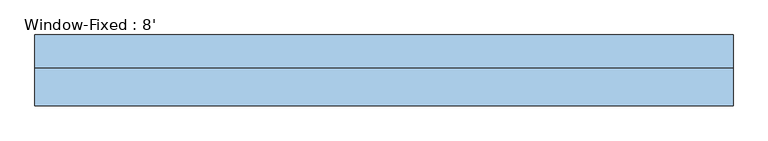
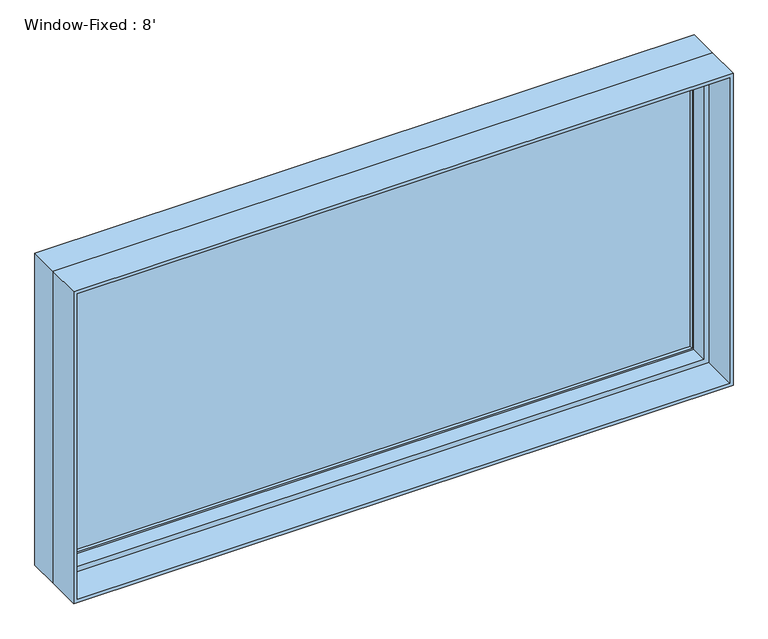
"""IFC4 building model written with IfcOpenShell, lengths in millimetres: window geometry, Window-Fixed : 8'."""

from ifc_helpers import new_model, si_unit, frame, origin, place, context, project, spatial, polyline, outline, extrude, faceted_brep, source, transform, mapped, element, save


def window_fixed_8_9704bb16(model_context):
    return source(origin(), model_context, "Body", "SolidModel", [
        faceted_brep([(1219.2, 19.05, 2133.6), (1219.2, 133.35, 2133.6), (-1219.2, 133.35, 2133.6), (-1219.2, 19.05, 2133.6), (-1219.2, 133.35, 914.4), (-1219.2, 19.05, 914.4), (1219.2, 133.35, 914.4), (1219.2, 19.05, 914.4), (1187.45, 19.05, 2101.85), (1187.45, 19.05, 946.15), (-1187.45, 19.05, 946.15), (-1187.45, 19.05, 2101.85), (-1206.5, 133.35, 2120.9), (-1206.5, 133.35, 927.1), (1206.5, 133.35, 927.1), (1206.5, 133.35, 2120.9), (1187.45, 82.55, 2101.85), (-1187.45, 82.55, 2101.85), (1206.5, 82.55, 2120.9), (-1206.5, 82.55, 2120.9), (-1187.45, 82.55, 946.15), (-1206.5, 82.55, 927.1), (1187.45, 82.55, 946.15), (1206.5, 82.55, 927.1)], [[[0, 1, 2, 3]], [[3, 2, 4, 5]], [[5, 4, 6, 7]], [[3, 5, 7, 0], [8, 9, 10, 11]], [[7, 6, 1, 0]], [[1, 6, 4, 2], [12, 13, 14, 15]], [[16, 8, 11, 17]], [[15, 18, 19, 12]], [[17, 11, 10, 20]], [[12, 19, 21, 13]], [[20, 10, 9, 22]], [[13, 21, 23, 14]], [[22, 9, 8, 16]], [[18, 23, 21, 19], [17, 20, 22, 16]], [[14, 23, 18, 15]]]),
        extrude(outline(polyline([(2133.6, -1219.2), (914.4, -1219.2), (914.4, 1219.2), (2133.6, 1219.2), (2133.6, -1219.2)]), holes=[polyline([(2120.9, 1206.5), (927.1, 1206.5), (927.1, -1206.5), (2120.9, -1206.5), (2120.9, 1206.5)])]), frame((0.0, -114.3, 0.0), z_axis=(0.0, 1.0, 0.0), x_axis=(0.0, 0.0, 1.0)), (0.0, 0.0, 1.0), 133.35),
        extrude(outline(polyline([(927.1, 1206.5), (2120.9, 1206.5), (2120.9, -1206.5), (927.1, -1206.5), (927.1, 1206.5)]), holes=[polyline([(952.5, -1181.1), (2095.5, -1181.1), (2095.5, 1181.1), (952.5, 1181.1), (952.5, -1181.1)])]), frame((0.0, 82.55, 0.0), z_axis=(0.0, 1.0, 0.0), x_axis=(0.0, 0.0, 1.0)), (0.0, 0.0, 1.0), 44.45),
        extrude(outline(polyline([(1181.1, 114.3), (1181.1, 107.95), (-1181.1, 107.95), (-1181.1, 114.3), (1181.1, 114.3)])), frame((0.0, 0.0, 952.5), z_axis=(0.0, 0.0, 1.0), x_axis=(1.0, 0.0, 0.0)), (0.0, 0.0, 1.0), 1143.0),
        extrude(outline(polyline([(-1181.1, 95.25), (-1181.1, 101.6), (1181.1, 101.6), (1181.1, 95.25), (-1181.1, 95.25)])), frame((0.0, 0.0, 952.5), z_axis=(0.0, 0.0, 1.0), x_axis=(1.0, 0.0, 0.0)), (0.0, 0.0, 1.0), 1143.0),
    ])


if __name__ == "__main__":
    model = new_model("IFC4")
    model_context = context("Model", 3, world=origin())
    ifc_project = project(units=[si_unit("LENGTHUNIT", "METRE", prefix="MILLI")], contexts=[model_context])
    site = spatial("IfcSite", under=ifc_project)
    building = spatial("IfcBuilding", under=site)
    placement = place(None, origin())
    window_fixed_8_shape = window_fixed_8_9704bb16(model_context)
    element("IfcWindow", 1, ObjectType="Window-Fixed : 8'", at=placement, inside=building, context=model_context, shape_type="MappedRepresentation", body=[
        mapped(window_fixed_8_shape, transform((0.0, 0.0, 0.0), x_axis=(1.0, 0.0, 0.0), y_axis=(0.0, 1.0, 0.0), z_axis=(0.0, 0.0, 1.0))),
    ])
    save(model, "model.ifc")

# Revit data of these elements
# Type "Window-Fixed : 8'"
#   Type Mark = "22"
#   Fire Rating = "0.5h"
#   Assembly Code = "B2020100"
#   Analytic Construction = "Double glazing - domestic"
#   Window Inset [instance default] = 0' - 0"
#   Wall Thickness [instance default] = 0' - 6"
#   Visual Light Transmittance = 0.81
#   Thermal Resistance (R) = 1.8146 (h·ft²·°F)/BTU
#   Solar Heat Gain Coefficient = 0.76
#   Rough Width = 8' - 0 1/2"
#   Rough Height = 4' - 0 1/2"
#   Interior Wall Closure [instance default] = 0' - 2 1/4"
#   Height = 4' - 0"
#   Heat Transfer Coefficient (U) = 0.5511 BTU/(h·ft²·°F)
#   Frame Extension [instance default] = 0' - 0 1/4"
#   Exterior Wall Closure [instance default] = 0' - 1 1/4"
#   Extension Jamb [instance default] = 0' - 2 1/4"
#   Default Sill Height = 3' - 0"
#   Width = 8' - 0"
#   Muntin Visibility = yes
#   Interior Trim Visibility [instance default] = yes
#   Exterior Trim Visibility [instance default] = yes
#   Extension Jamb Visibility [instance default] = yes
#   Muntin Pattern = Muntin Pattern_2x2 : Muntin Pattern_2x2
#   Interior Trim Material = Wood - Stained
#   Interior Trim = Trim-Window-Interior-Flat : Picture Frame
#   Interior Frame Material = Wood - Stained
#   Glass Panel Material = Glass
#   Exterior Trim Material = Clad - White
#   Exterior Trim = Trim-Window-Exterior-Flat : with Sill
#   Exterior Frame Material = Clad - White
#   Wall Closure = (empty or 0)
# Element 1 (IfcWindow, "Window-Fixed : 8'")
#   Wall Thickness = 0' - 9"
#   Extension Jamb = 0' - 5 1/4"
#   Materials on its faces: "Wood - Stained", "Glass", "Clad - White"
# Materials
#   "Wood - Stained": class "Wood", colour RGB 224 178 126, transparency 0, Cost = 0
#   "Glass": class "Glass", colour RGB 0 128 192, transparency 0.75, Description = "Soda Lime Glass", Cost = 0
#   "Clad - White": class "Wood", colour RGB 242 242 238, transparency 0, Cost = 0
